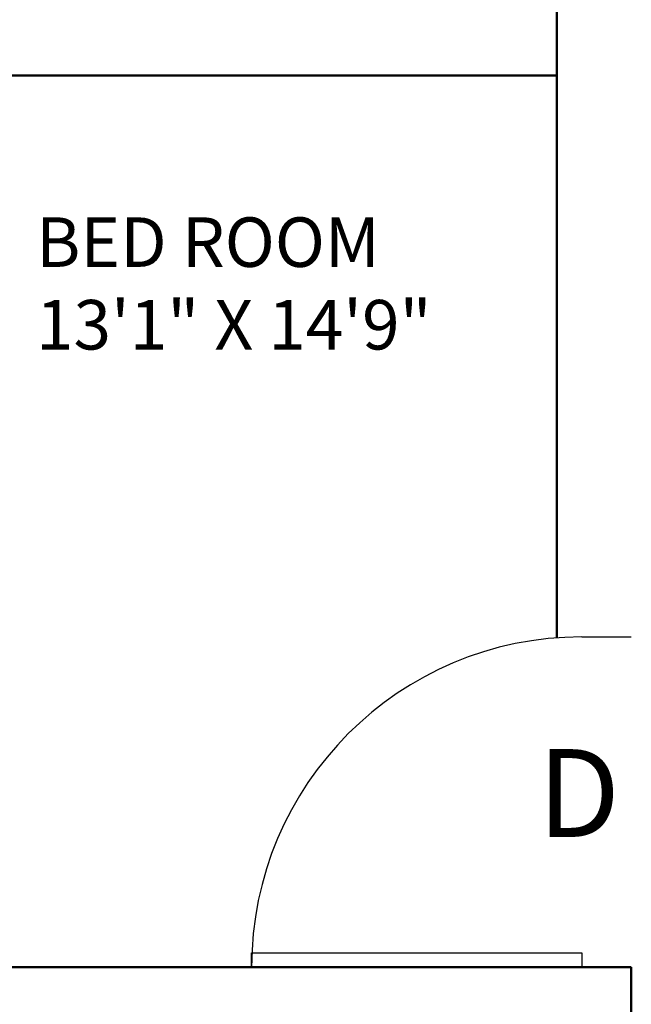
# Model space of a CAD drawing. Units: inches. Extents: x -105 to 1196, y -792 to 119.
# Tile 8 of 23: x 56 to 130, y -121 to -1. Entities that reach past the tile are written whole.
import ezdxf

# ---------------------------------------------------------------- set-up
doc = ezdxf.new("R2010")
doc.units = ezdxf.units.IN
doc.header["$MEASUREMENT"] = 0
for name, color, linetype, lineweight in [('A-ANNO-TEXT', 7, 'Continuous', 25), ('A-AREA-IDEN', 7, 'Continuous', 25), ('A-DOOR', 4, 'Continuous', 25), ('A-WALL', 3, 'Continuous', 50)]:
    doc.layers.add(name, color=color, linetype=linetype, lineweight=lineweight)
doc.styles.get("Standard").update_dxf_attribs({"font": 'arial.ttf'})

# ---------------------------------------------------------------- blocks, each defined once
blk = doc.blocks.new('*U4')
for p, q in [((0, 0), (0, -6)), ((40, 0), (40, -6))]:
    blk.add_line(p, q)
blk.add_lwpolyline([(0, 0), (0, 40), (1.75, 40), (1.75, 0)], close=True)
blk.add_arc((0, 0), 40, 0, 90)

msp = doc.modelspace()

# ---------------------------------------------------------------- linework, layer by layer
at = {"layer": 'A-WALL'}
for p, q in [((120.74, 60.77), (120.74, -76.34)), ((120.74, -8.23), (48.74, -8.23)), ((-36.26, -116.23), (129.74, -116.23)), ((129.74, -116.23), (129.74, -242.23))]:
    msp.add_line(p, q, dxfattribs=at)

# ---------------------------------------------------------------- block references
at = {"layer": 'A-DOOR', "rotation": 90}
msp.add_blockref('*U4', (123.74, -116.23), dxfattribs=at)

# ---------------------------------------------------------------- texts
at = {"layer": 'A-ANNO-TEXT'}
msp.add_text('D', height=10.64, dxfattribs=at).set_placement((118.4, -100.46))
at = {"layer": 'A-AREA-IDEN', "insert": (57.62, -25.42), "char_height": 6, "attachment_point": 1}
msp.add_mtext_dynamic_manual_height_columns('BED ROOM\\P13\'1" X 14\'9"', width=59.5623, gutter_width=1, heights=[0], dxfattribs=at)

doc.saveas('drawing.dxf')
